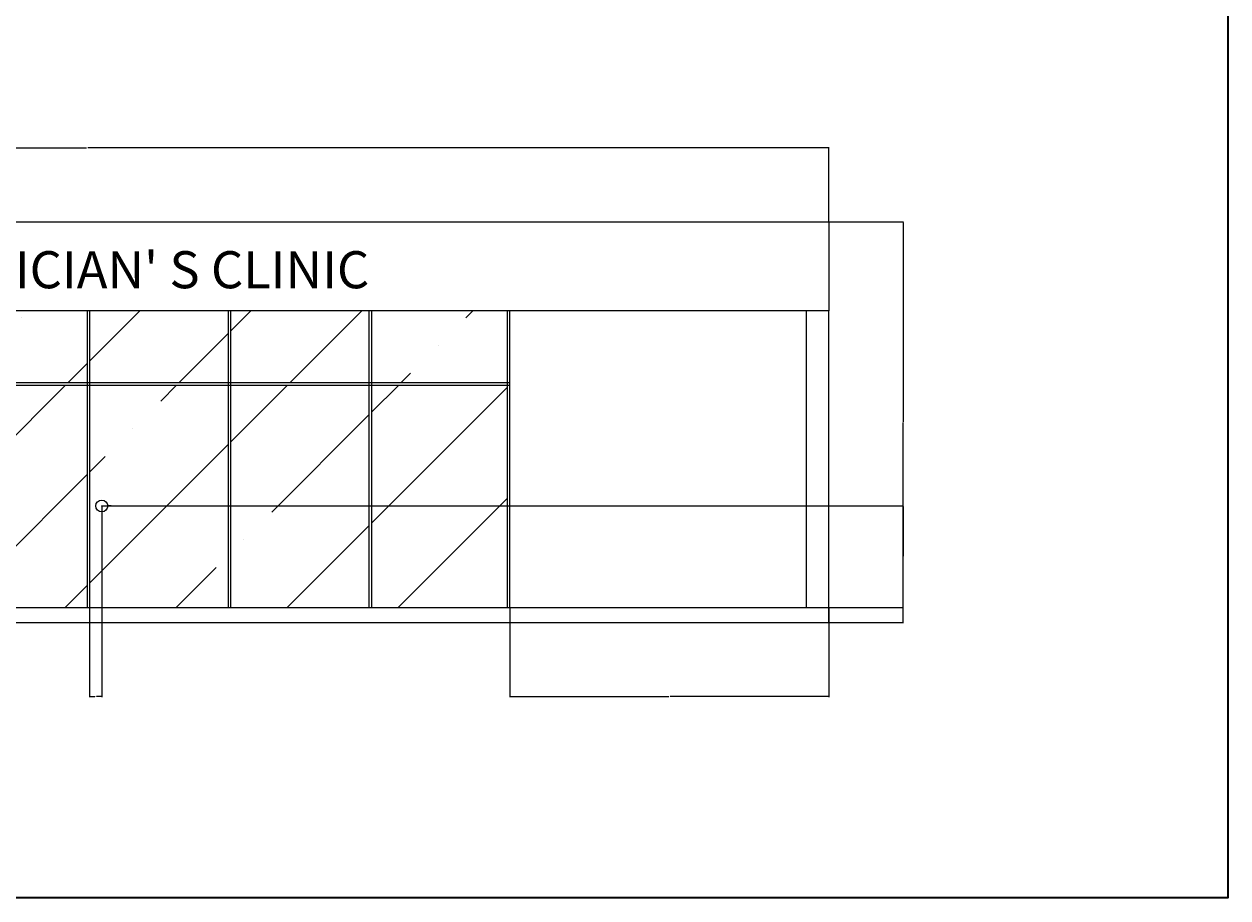
# Model space of a CAD drawing. Units: inches. Extents: x 7245 to 8143, y 15548 to 17244.
# Tile 2 of 5: x 7657 to 8143, y 15548 to 15902. Entities that reach past the tile are written whole.
import ezdxf

# ---------------------------------------------------------------- set-up
doc = ezdxf.new("R2010")
doc.units = ezdxf.units.IN
for name, color, linetype, lineweight in [('A-ANNO-DIMS', 2, 'Continuous', 18), ('A-ANNO-TEXT', 7, 'Continuous', 25), ('A-ANNO-TTLB', 7, 'Continuous', 35), ('A-ELEV', 7, 'Continuous', 25), ('A-ELEV-GLAZ', 4, 'Continuous', 18), ('A-ELEV-PATT', 252, 'Continuous', 13)]:
    doc.layers.add(name, color=color, linetype=linetype, lineweight=lineweight)
doc.styles.get("Standard").update_dxf_attribs({"font": 'arial.ttf'})
doc.dimstyles.get("Standard").update_dxf_attribs({"dimtxt": 0.18, "dimasz": 0.18, "dimexe": 0.18, "dimexo": 0.0625, "dimgap": 0.09, "dimtad": 0, "dimtih": 1, "dimtoh": 1, "dimdec": 4, "dimzin": 0, "dimdsep": 46, "dimtxsty": 'Standard', "dimcen": 0.09, "dimadec": 0, "dimazin": 0, "dimtfac": 1, "dimtdec": 4, "dimtofl": 0, "dimtmove": 0, "dimatfit": 3, "dimfxl": 1, "dimtolj": 1, "dimtzin": 0, "dimarcsym": 0})

# ---------------------------------------------------------------- blocks, each defined once
blk = doc.blocks.new('*D69')
at = {"layer": 'A-ANNO-DIMS', "color": 0, "lineweight": -2, "transparency": 16777216}
for p, q in [((7382.08, 15821.68), (7382.08, 15851.81)), ((7382.26, 15851.63), (7681.79, 15851.63)), ((7981.9, 15851.63), (7682.37, 15851.63)), ((7982.08, 15821.68), (7982.08, 15851.81))]:
    blk.add_line(p, q, dxfattribs=at)
at = {"layer": 'A-ANNO-DIMS', "color": 0, "transparency": 16777216}
for points in [[(7382.26, 15851.66), (7382.26, 15851.6), (7382.08, 15851.63)], [(7981.9, 15851.66), (7981.9, 15851.6), (7982.08, 15851.63)]]:
    blk.add_solid(points, dxfattribs=at)
at = {"layer": 'Defpoints', "color": 0, "transparency": 16777216}
for p in [(7982.08, 15851.63), (7382.08, 15821.62), (7982.08, 15821.62)]:
    blk.add_point(p, dxfattribs=at)
at = {"layer": 'A-ANNO-DIMS', "color": 0, "transparency": 16777216, "insert": (7682.08, 15851.63), "char_height": 0.18, "attachment_point": 5}
blk.add_mtext('\\A1;600', dxfattribs=at)
blk = doc.blocks.new('*D70')
at = {"layer": 'A-ANNO-DIMS', "color": 0, "lineweight": -2, "transparency": 16777216}
for p, q in [((7982.15, 15821.62), (8012.28, 15821.62)), ((8012.1, 15821.44), (8012.1, 15740.8)), ((8012.1, 15659.8), (8012.1, 15740.44)), ((7982.15, 15659.62), (8012.28, 15659.62))]:
    blk.add_line(p, q, dxfattribs=at)
at = {"layer": 'A-ANNO-DIMS', "color": 0, "transparency": 16777216}
for points in [[(8012.07, 15821.44), (8012.13, 15821.44), (8012.1, 15821.62)], [(8012.07, 15659.8), (8012.13, 15659.8), (8012.1, 15659.62)]]:
    blk.add_solid(points, dxfattribs=at)
at = {"layer": 'Defpoints', "color": 0, "transparency": 16777216}
for p in [(7982.08, 15821.62), (8012.1, 15821.62), (7982.08, 15659.62)]:
    blk.add_point(p, dxfattribs=at)
at = {"layer": 'A-ANNO-DIMS', "color": 0, "transparency": 16777216, "insert": (8012.1, 15740.62), "char_height": 0.18, "attachment_point": 5}
blk.add_mtext('\\A1;162', dxfattribs=at)
blk = doc.blocks.new('*D73')
at = {"layer": 'A-ANNO-DIMS', "color": 0, "lineweight": -2, "transparency": 16777216}
for p, q in [((7853.08, 15665.56), (7853.08, 15629.42)), ((7982.08, 15665.56), (7982.08, 15629.42)), ((7853.26, 15629.6), (7917.3, 15629.6)), ((7981.9, 15629.6), (7917.86, 15629.6))]:
    blk.add_line(p, q, dxfattribs=at)
at = {"layer": 'A-ANNO-DIMS', "color": 0, "transparency": 16777216}
for points in [[(7853.26, 15629.63), (7853.26, 15629.57), (7853.08, 15629.6)], [(7981.9, 15629.63), (7981.9, 15629.57), (7982.08, 15629.6)]]:
    blk.add_solid(points, dxfattribs=at)
at = {"layer": 'Defpoints', "color": 0, "transparency": 16777216}
for p in [(7853.08, 15665.62), (7982.08, 15665.62), (7982.08, 15629.6)]:
    blk.add_point(p, dxfattribs=at)
at = {"layer": 'A-ANNO-DIMS', "color": 0, "transparency": 16777216, "insert": (7917.58, 15629.6), "char_height": 0.18, "attachment_point": 5}
blk.add_mtext('\\A1;129', dxfattribs=at)
blk = doc.blocks.new('*D77')
at = {"layer": 'A-ANNO-DIMS', "color": 0, "lineweight": -2, "transparency": 16777216}
for p, q in [((7688.05, 15706.71), (8012.28, 15706.71)), ((8012.1, 15706.53), (8012.1, 15686.34)), ((8012.1, 15665.8), (8012.1, 15685.98)), ((7683.15, 15665.62), (8012.28, 15665.62))]:
    blk.add_line(p, q, dxfattribs=at)
at = {"layer": 'A-ANNO-DIMS', "color": 0, "transparency": 16777216}
for points in [[(8012.07, 15706.53), (8012.13, 15706.53), (8012.1, 15706.71)], [(8012.07, 15665.8), (8012.13, 15665.8), (8012.1, 15665.62)]]:
    blk.add_solid(points, dxfattribs=at)
at = {"layer": 'Defpoints', "color": 0, "transparency": 16777216}
for p in [(7687.99, 15706.71), (7683.08, 15665.62), (8012.1, 15665.62)]:
    blk.add_point(p, dxfattribs=at)
at = {"layer": 'A-ANNO-DIMS', "color": 0, "transparency": 16777216, "insert": (8012.1, 15686.16), "char_height": 0.18, "attachment_point": 5}
blk.add_mtext('\\A1;41.09', dxfattribs=at)
blk = doc.blocks.new('*D78')
at = {"layer": 'A-ANNO-DIMS', "color": 0, "lineweight": -2, "transparency": 16777216}
for p, q in [((7687.99, 15706.64), (7687.99, 15629.42)), ((7683.08, 15665.56), (7683.08, 15629.42)), ((7683.26, 15629.6), (7685.14, 15629.6)), ((7687.81, 15629.6), (7685.94, 15629.6))]:
    blk.add_line(p, q, dxfattribs=at)
at = {"layer": 'A-ANNO-DIMS', "color": 0, "transparency": 16777216}
for points in [[(7683.26, 15629.63), (7683.26, 15629.57), (7683.08, 15629.6)], [(7687.81, 15629.63), (7687.81, 15629.57), (7687.99, 15629.6)]]:
    blk.add_solid(points, dxfattribs=at)
at = {"layer": 'Defpoints', "color": 0, "transparency": 16777216}
for p in [(7687.99, 15706.71), (7683.08, 15665.62), (7687.99, 15629.6)]:
    blk.add_point(p, dxfattribs=at)
at = {"layer": 'A-ANNO-DIMS', "color": 0, "transparency": 16777216, "insert": (7685.54, 15629.6), "char_height": 0.18, "attachment_point": 5}
blk.add_mtext('\\A1;4.908', dxfattribs=at)
blk = doc.blocks.new('*D83')
at = {"layer": 'A-ANNO-DIMS', "color": 0, "lineweight": -2, "transparency": 16777216}
for p, q in [((7687.9, 15706.71), (7688.08, 15706.71)), ((7687.99, 15706.62), (7687.99, 15706.8)), ((7691.86, 15706.76), (7690.59, 15706.74))]:
    blk.add_line(p, q, dxfattribs=at)
at = {"layer": 'A-ANNO-DIMS', "color": 0, "transparency": 16777216}
blk.add_solid([(7690.59, 15706.77), (7690.59, 15706.71), (7690.41, 15706.74)], dxfattribs=at)
at = {"layer": 'Defpoints', "color": 0, "transparency": 16777216}
for p in [(7685.58, 15706.67), (7690.41, 15706.74)]:
    blk.add_point(p, dxfattribs=at)
at = {"layer": 'A-ANNO-DIMS', "color": 0, "transparency": 16777216, "insert": (7692.35, 15706.76), "char_height": 0.18, "attachment_point": 5}
blk.add_mtext('\\A1;∅4.833', dxfattribs=at)

msp = doc.modelspace()

# ---------------------------------------------------------------- hatches: boundary and pattern name
at = {"layer": 'A-ELEV-PATT'}
h = msp.add_hatch(dxfattribs=at)
h.set_pattern_fill('ANSI35', color=256, scale=10)
h.paths.add_polyline_path([(7568.0838, 15755.6176), (7512.0838, 15755.6176), (7512.0838, 15665.6176), (7568.0838, 15665.6176)])
h.paths.add_polyline_path([(7568.0838, 15785.6176), (7512.0838, 15785.6176), (7512.0838, 15756.6176), (7568.0838, 15756.6176)])
h.paths.add_polyline_path([(7625.0838, 15785.6176), (7569.0838, 15785.6176), (7569.0838, 15756.6176), (7625.0838, 15756.6176)])
h.paths.add_polyline_path([(7625.0838, 15755.6176), (7569.0838, 15755.6176), (7569.0838, 15665.6176), (7625.0838, 15665.6176)])
h.paths.add_polyline_path([(7682.0838, 15755.6176), (7626.0838, 15755.6176), (7626.0838, 15665.6176), (7682.0838, 15665.6176)])
h.paths.add_polyline_path([(7682.0838, 15785.6176), (7626.0838, 15785.6176), (7626.0838, 15756.6176), (7682.0838, 15756.6176)])
h.paths.add_polyline_path([(7739.0838, 15785.6176), (7683.0838, 15785.6176), (7683.0838, 15756.6176), (7739.0838, 15756.6176)])
h.paths.add_polyline_path([(7796.0838, 15785.6176), (7740.0838, 15785.6176), (7740.0838, 15756.6176), (7796.0838, 15756.6176)])
h.paths.add_polyline_path([(7852.0838, 15785.6176), (7797.0838, 15785.6176), (7797.0838, 15756.6176), (7852.0838, 15756.6176)])
h.paths.add_polyline_path([(7852.0838, 15755.6176), (7797.0838, 15755.6176), (7797.0838, 15665.6176), (7852.0838, 15665.6176)])
h.paths.add_polyline_path([(7796.0838, 15755.6176), (7740.0838, 15755.6176), (7740.0838, 15665.6176), (7796.0838, 15665.6176)])
h.paths.add_polyline_path([(7739.0838, 15755.6176), (7683.0838, 15755.6176), (7683.0838, 15665.6176), (7739.0838, 15665.6176)])
h.paths.add_polyline_path([(7690.4084, 15706.7064, -1), (7685.5756, 15706.7064, -1)], flags=16)

# ---------------------------------------------------------------- linework, layer by layer
at = {"layer": 'A-ANNO-TTLB'}
msp.add_lwpolyline([(7245.2864, 17243.9412), (8143.486, 17243.9412), (8143.486, 15548.1459), (7245.2864, 15548.1459)], close=True, dxfattribs=at)
at = {"layer": 'A-ELEV'}
for p, q in [((7382.0838, 15821.6176), (7982.0838, 15821.6176)), ((7982.0838, 15821.6176), (7982.0838, 15785.6176)), ((7982.0838, 15785.6176), (7382.0838, 15785.6176)), ((7973.0838, 15665.6176), (7973.0838, 15785.6176)), ((7982.0838, 15665.6176), (7982.0838, 15785.6176)), ((7382.0838, 15665.6176), (7982.0838, 15665.6176)), ((7982.0838, 15659.6176), (7982.0838, 15665.6176)), ((7382.0838, 15659.6176), (7982.0838, 15659.6176))]:
    msp.add_line(p, q, dxfattribs=at)
at = {"layer": 'A-ELEV-GLAZ'}
for p, q in [((7682.0838, 15785.6176), (7682.0838, 15665.6176)), ((7683.0838, 15785.6176), (7683.0838, 15665.6176)), ((7739.0838, 15785.6176), (7739.0838, 15665.6176)), ((7740.0838, 15785.6176), (7740.0838, 15665.6176)), ((7796.0838, 15785.6176), (7796.0838, 15665.6176)), ((7797.0838, 15785.6176), (7797.0838, 15665.6176)), ((7852.0838, 15665.6176), (7852.0838, 15785.6176)), ((7853.0838, 15665.6176), (7853.0838, 15785.6176)), ((7511.0838, 15756.6176), (7853.0838, 15756.6176)), ((7511.0838, 15755.6176), (7853.0838, 15755.6176))]:
    msp.add_line(p, q, dxfattribs=at)
msp.add_circle((7687.992, 15706.7064), 2.4164, dxfattribs=at)

# ---------------------------------------------------------------- texts
at = {"layer": 'A-ANNO-TEXT', "insert": (7583.1007, 15809.7842), "char_height": 15, "attachment_point": 1}
msp.add_mtext_dynamic_manual_height_columns("\\pxqc;{\\fArial|b1|i0|c0|p34;PHYSICIAN' S CLINIC}", width=231.895772, gutter_width=18.8458, heights=[0], dxfattribs=at)

# ---------------------------------------------------------------- dimensions: what is measured, and where the dimension line sits
at = {"layer": 'A-ANNO-DIMS'}
for base, p1, p2, override, picture, middle in [((7982.0838, 15851.6326), (7382.0838, 15821.6176), (7982.0838, 15821.6176), {"dimdec": 0, "dimlfac": 1, "dimrnd": 0, "dimzin": 0, "dimdsep": 46, "dimlunit": 2}, '*D69', (7682.0838, 15851.6326)), ((7687.992, 15629.6027), (7683.0838, 15665.6176), (7687.992, 15706.7064), {"dimdec": 3, "dimlfac": 1, "dimrnd": 0, "dimzin": 0, "dimdsep": 46, "dimlunit": 2}, '*D78', (7685.5379, 15629.6027)), ((7982.0838, 15629.6027), (7853.0838, 15665.6176), (7982.0838, 15665.6176), {"dimdec": 0, "dimlfac": 1, "dimrnd": 0, "dimzin": 0, "dimdsep": 46, "dimlunit": 2}, '*D73', (7917.5838, 15629.6027))]:
    dim = msp.add_linear_dim(base=base, p1=p1, p2=p2, dimstyle='Standard', override=override, dxfattribs=at)
    dim.commit()
    dim.dimension.update_dxf_attribs({"geometry": picture, "text_midpoint": middle})
for base, p1, p2, override, picture, middle in [((8012.0988, 15821.6176), (7982.0838, 15659.6176), (7982.0838, 15821.6176), {"dimdec": 0, "dimlfac": 1, "dimrnd": 0, "dimzin": 0, "dimdsep": 46, "dimlunit": 2}, '*D70', (8012.0988, 15740.6177)), ((8012.0988, 15665.6176), (7687.992, 15706.7064), (7683.0838, 15665.6176), {"dimdec": 2, "dimlfac": 1, "dimrnd": 0, "dimzin": 0, "dimdsep": 46, "dimlunit": 2}, '*D77', (8012.0988, 15686.162))]:
    dim = msp.add_linear_dim(base=base, p1=p1, p2=p2, angle=90, dimstyle='Standard', override=override, dxfattribs=at)
    dim.commit()
    dim.dimension.update_dxf_attribs({"geometry": picture, "text_midpoint": middle})
dim = msp.add_diameter_dim_2p(p1=(7685.5759, 15706.6722), p2=(7690.4082, 15706.7405), dimstyle='Standard', override={"dimdec": 3, "dimlfac": 1, "dimrnd": 0, "dimzin": 0, "dimdsep": 46, "dimlunit": 2}, dxfattribs=at)
dim.commit()
dim.dimension.update_dxf_attribs({"geometry": '*D83', "text_midpoint": (7691.8579, 15706.761), "dimtype": 163})

doc.saveas('drawing.dxf')
